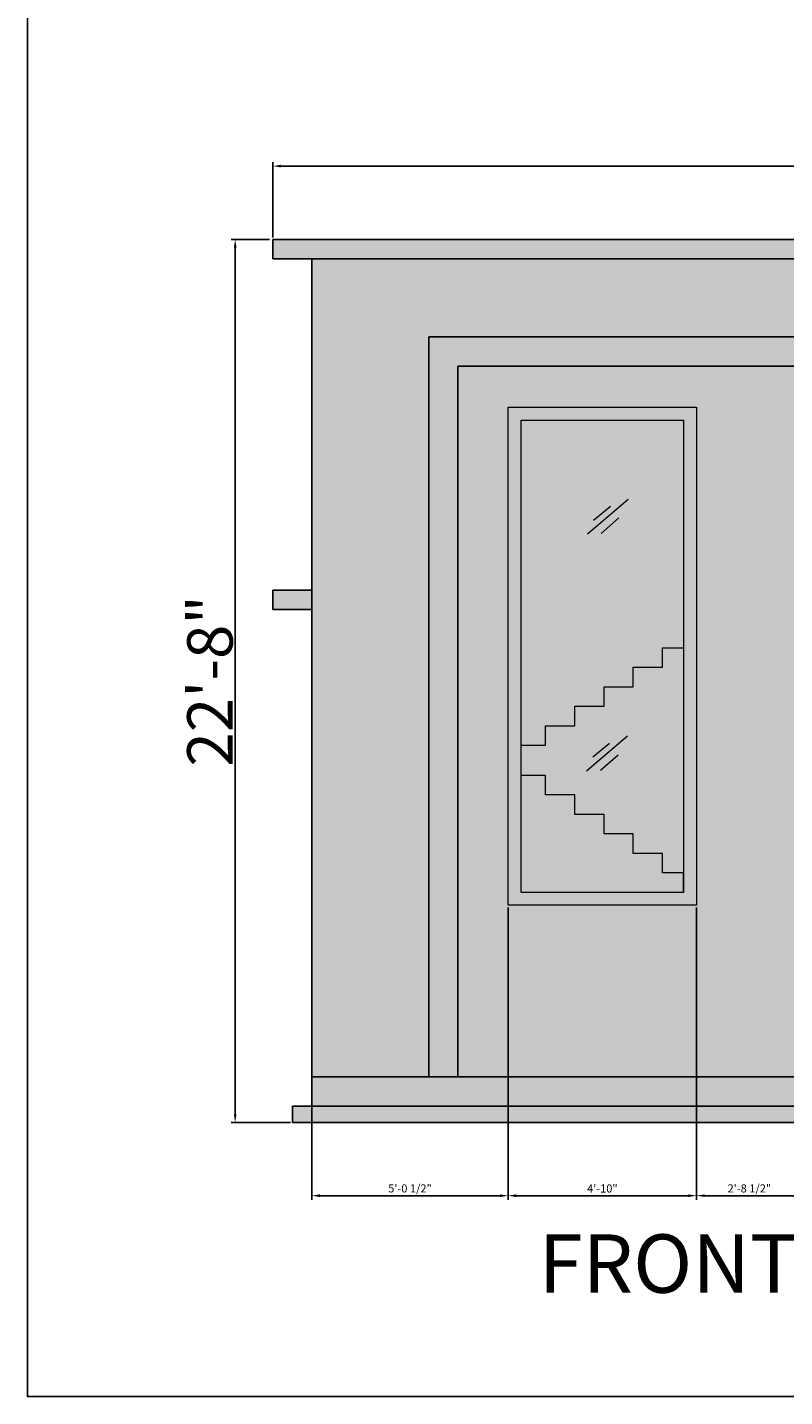
# Model space of a CAD drawing. Units: inches. Extents: x 2169 to 10664, y 1669 to 6352.
# Tile 1 of 17: x 2169 to 2403, y 1669 to 2091. Entities that reach past the tile are written whole.
import ezdxf

# ---------------------------------------------------------------- set-up
doc = ezdxf.new("R2010")
doc.units = ezdxf.units.IN
for name, color, linetype, lineweight in [('A-ANNO-DIMS', 3, 'Continuous', 18), ('A-ANNO-TITL', 3, 'Continuous', 25), ('A-ANNO-TTLB', 7, 'Continuous', 25), ('A-ELEV', 7, 'Continuous', 25), ('A-ELEV-CONC-PATT', 85, 'Continuous', 13), ('A-ELEV-OPEN', 7, 'Continuous', 18), ('A-ELEV-OPEN-PATT', 9, 'Continuous', 13), ('A-ELEV-PATT', 253, 'Continuous', 13), ('A-ELEV-STRS', 8, 'Continuous', 18)]:
    doc.layers.add(name, color=color, linetype=linetype, lineweight=lineweight)
doc.styles.get("Standard").update_dxf_attribs({"font": 'arial.ttf'})
doc.dimstyles.new('ISO-25', dxfattribs={"dimtxt": 2.5, "dimasz": 2.5, "dimexe": 1.25, "dimexo": 0.625, "dimtad": 1, "dimdec": 0, "dimlunit": 3, "dimtxsty": 'Standard', "dimcen": 2.5, "dimadec": 0, "dimazin": 0, "dimtfac": 1, "dimtdec": 0, "dimtmove": 0, "dimatfit": 3, "dimfxl": 1, "dimarcsym": 0})

# ---------------------------------------------------------------- blocks, each defined once
blk = doc.blocks.new('*D21')
at = {"layer": 'A-ANNO-DIMS', "color": 0, "lineweight": -2, "transparency": 16777216}
for p, q in [((2243.98, 2025.84), (2232.19, 2025.84)), ((2233.44, 2023.34), (2233.44, 1756.34)), ((2250.43, 1753.84), (2232.19, 1753.84))]:
    blk.add_line(p, q, dxfattribs=at)
at = {"layer": 'A-ANNO-DIMS', "color": 0, "transparency": 16777216}
for points in [[(2233.03, 2023.34), (2233.86, 2023.34), (2233.44, 2025.84)], [(2233.03, 1756.34), (2233.86, 1756.34), (2233.44, 1753.84)]]:
    blk.add_solid(points, dxfattribs=at)
at = {"layer": 'Defpoints', "color": 0, "transparency": 16777216}
for p in [(2244.61, 2025.84), (2233.44, 1753.84), (2251.06, 1753.84)]:
    blk.add_point(p, dxfattribs=at)
at = {"layer": 'A-ANNO-DIMS', "color": 0, "transparency": 16777216, "insert": (2225.67, 1889.84), "char_height": 2.5, "attachment_point": 5, "rotation": 90}
blk.add_mtext('{\\H5.6x;22\'-8"}', dxfattribs=at)
blk = doc.blocks.new('GLASS-MARK-A')
for p, q in [((0, 0), (12.55, 10.69)), ((1.85, 4.25), (7.07, 8.47)), ((4.25, 0.12), (9.7, 4.88))]:
    blk.add_line(p, q)
blk = doc.blocks.new('*D93')
at = {"layer": 'A-ANNO-DIMS', "color": 0, "lineweight": -2, "transparency": 16777216}
for p, q in [((2245.06, 2026.47), (2245.06, 2049.69)), ((2247.56, 2048.44), (2626.56, 2048.44)), ((2629.06, 2026.47), (2629.06, 2049.69))]:
    blk.add_line(p, q, dxfattribs=at)
at = {"layer": 'A-ANNO-DIMS', "color": 0, "transparency": 16777216}
for points in [[(2247.56, 2048.86), (2247.56, 2048.03), (2245.06, 2048.44)], [(2626.56, 2048.86), (2626.56, 2048.03), (2629.06, 2048.44)]]:
    blk.add_solid(points, dxfattribs=at)
at = {"layer": 'Defpoints', "color": 0, "transparency": 16777216}
for p in [(2629.06, 2048.44), (2245.06, 2025.84), (2629.06, 2025.84)]:
    blk.add_point(p, dxfattribs=at)
at = {"layer": 'A-ANNO-DIMS', "color": 0, "transparency": 16777216, "insert": (2437.06, 2050.35), "char_height": 2.5, "attachment_point": 5}
blk.add_mtext('32\'-0"', dxfattribs=at)
blk = doc.blocks.new('*D95')
at = {"layer": 'A-ANNO-DIMS', "color": 0, "lineweight": -2, "transparency": 16777216}
for p, q in [((2317.5, 1820.07), (2317.5, 1729.99)), ((2257.06, 1767.22), (2257.06, 1729.99)), ((2259.56, 1731.24), (2315, 1731.24))]:
    blk.add_line(p, q, dxfattribs=at)
at = {"layer": 'A-ANNO-DIMS', "color": 0, "transparency": 16777216}
for points in [[(2259.56, 1731.66), (2259.56, 1730.83), (2257.06, 1731.24)], [(2315, 1731.66), (2315, 1730.83), (2317.5, 1731.24)]]:
    blk.add_solid(points, dxfattribs=at)
at = {"layer": 'Defpoints', "color": 0, "transparency": 16777216}
for p in [(2317.5, 1820.7), (2257.06, 1767.84), (2317.5, 1731.24)]:
    blk.add_point(p, dxfattribs=at)
at = {"layer": 'A-ANNO-DIMS', "color": 0, "transparency": 16777216, "insert": (2287.28, 1733.16), "char_height": 2.5, "attachment_point": 5}
blk.add_mtext('5\'-0 1/2"', dxfattribs=at)
blk = doc.blocks.new('*D96')
at = {"layer": 'A-ANNO-DIMS', "color": 0, "lineweight": -2, "transparency": 16777216}
for p, q in [((2317.5, 1820.07), (2317.5, 1729.99)), ((2375.55, 1820.07), (2375.55, 1729.99)), ((2320, 1731.24), (2373.05, 1731.24))]:
    blk.add_line(p, q, dxfattribs=at)
at = {"layer": 'A-ANNO-DIMS', "color": 0, "transparency": 16777216}
for points in [[(2320, 1731.66), (2320, 1730.83), (2317.5, 1731.24)], [(2373.05, 1731.66), (2373.05, 1730.83), (2375.55, 1731.24)]]:
    blk.add_solid(points, dxfattribs=at)
at = {"layer": 'Defpoints', "color": 0, "transparency": 16777216}
for p in [(2317.5, 1820.7), (2375.55, 1820.7), (2375.55, 1731.24)]:
    blk.add_point(p, dxfattribs=at)
at = {"layer": 'A-ANNO-DIMS', "color": 0, "transparency": 16777216, "insert": (2346.52, 1733.14), "char_height": 2.5, "attachment_point": 5}
blk.add_mtext('4\'-10"', dxfattribs=at)
blk = doc.blocks.new('*D97')
at = {"layer": 'A-ANNO-DIMS', "color": 0, "lineweight": -2, "transparency": 16777216}
for p, q in [((2375.55, 1820.07), (2375.55, 1729.99)), ((2408.06, 1767.22), (2408.06, 1729.99)), ((2378.05, 1731.24), (2405.56, 1731.24))]:
    blk.add_line(p, q, dxfattribs=at)
at = {"layer": 'A-ANNO-DIMS', "color": 0, "transparency": 16777216}
for points in [[(2378.05, 1731.66), (2378.05, 1730.83), (2375.55, 1731.24)], [(2405.56, 1731.66), (2405.56, 1730.83), (2408.06, 1731.24)]]:
    blk.add_solid(points, dxfattribs=at)
at = {"layer": 'Defpoints', "color": 0, "transparency": 16777216}
for p in [(2375.55, 1820.7), (2408.06, 1767.84), (2408.06, 1731.24)]:
    blk.add_point(p, dxfattribs=at)
at = {"layer": 'A-ANNO-DIMS', "color": 0, "transparency": 16777216, "insert": (2391.8, 1733.16), "char_height": 2.5, "attachment_point": 5}
blk.add_mtext('2\'-8 1/2"', dxfattribs=at)

msp = doc.modelspace()

# ---------------------------------------------------------------- hatches: boundary and pattern name
at = {"layer": 'A-ELEV-CONC-PATT'}
h = msp.add_hatch(dxfattribs=at)
h.set_pattern_fill('AR-CONC', color=256, scale=0.02)
h.paths.add_polyline_path([(2629.06, 2025.84), (2245.06, 2025.84), (2245.06, 2019.84), (2629.06, 2019.84)])
h.paths.add_polyline_path([(2257.06, 1917.84), (2245.06, 1917.84), (2245.06, 1911.84), (2257.06, 1911.84)])
h.paths.add_polyline_path([(2629.06, 1917.84), (2408.06, 1917.84), (2408.06, 1911.84), (2629.06, 1911.84)])
h = msp.add_hatch(dxfattribs=at)
h.set_pattern_fill('AR-CONC', color=256, scale=0.02)
h.paths.add_polyline_path([(2408.06, 1995.84), (2293.06, 1995.84), (2293.06, 1767.84), (2302.06, 1767.84), (2302.06, 1986.84), (2408.06, 1986.84)])
at = {"layer": 'A-ELEV-OPEN-PATT'}
h = msp.add_hatch(color=256, dxfattribs=at)
h.dxf.hatch_style = 1
h.paths.add_polyline_path([(2375.55, 1974.13), (2317.5, 1974.13), (2317.5, 1820.7), (2375.55, 1820.7)])
h.paths.add_polyline_path([(2371.55, 1970.13), (2371.55, 1824.7), (2321.5, 1824.7), (2321.5, 1970.13)], flags=16)
h = msp.add_hatch(color=256, dxfattribs=at)
h.dxf.hatch_style = 1
h.paths.add_polyline_path([(2608.06, 1955.84), (2408.06, 1955.84), (2408.06, 1923.84), (2608.06, 1923.84)])
h.paths.add_polyline_path([(2371.55, 1970.13), (2321.5, 1970.13), (2321.5, 1870.03), (2329.06, 1870.03), (2329.06, 1876.03), (2338.06, 1876.03), (2338.06, 1882.03), (2347.06, 1882.03), (2347.06, 1888.03), (2356.06, 1888.03), (2356.06, 1894.03), (2365.06, 1894.03), (2365.06, 1900.03), (2371.55, 1900.03)])
h.paths.add_polyline_path([(2371.55, 1900.03), (2365.06, 1900.03), (2365.06, 1894.03), (2356.06, 1894.03), (2356.06, 1888.03), (2347.06, 1888.03), (2347.06, 1882.03), (2338.06, 1882.03), (2338.06, 1876.03), (2329.06, 1876.03), (2329.06, 1870.03), (2321.5, 1870.03), (2321.5, 1860.7), (2329.06, 1860.7), (2329.06, 1854.7), (2338.06, 1854.7), (2338.06, 1848.7), (2347.06, 1848.7), (2347.06, 1842.7), (2356.06, 1842.7), (2356.06, 1836.7), (2365.06, 1836.7), (2365.06, 1830.7), (2371.55, 1830.7)])
h.paths.add_polyline_path([(2365.06, 1836.7), (2356.06, 1836.7), (2356.06, 1842.7), (2347.06, 1842.7), (2347.06, 1848.7), (2338.06, 1848.7), (2338.06, 1854.7), (2329.06, 1854.7), (2329.06, 1860.7), (2321.5, 1860.7), (2321.5, 1824.7), (2371.55, 1824.7), (2371.55, 1830.7), (2365.06, 1830.7)])
at = {"layer": 'A-ELEV-PATT'}
h = msp.add_hatch(color=256, dxfattribs=at)
h.dxf.hatch_style = 1
h.paths.add_polyline_path([(2408.06, 1986.84), (2302.06, 1986.84), (2302.06, 1767.84), (2408.06, 1767.84)], flags=17)
h.paths.add_polyline_path([(2375.55, 1820.7), (2317.5, 1820.7), (2317.5, 1974.13), (2375.55, 1974.13)], flags=16)
h.paths.add_polyline_path([(2371.55, 1824.7), (2321.5, 1824.7), (2321.5, 1970.13), (2371.55, 1970.13)], flags=0)
h.paths.add_polyline_path([(2293.06, 1995.84), (2408.06, 1995.84), (2408.06, 2019.84), (2257.06, 2019.84), (2257.06, 1767.84), (2293.06, 1767.84)])
h = msp.add_hatch(color=256, dxfattribs=at)
h.dxf.hatch_style = 1
h.paths.add_polyline_path([(2617.06, 1767.84), (2257.06, 1767.84), (2257.06, 1758.84), (2617.06, 1758.84)])
h = msp.add_hatch(color=256, dxfattribs=at)
h.dxf.hatch_style = 1
h.paths.add_polyline_path([(2623.06, 1758.84), (2251.06, 1758.84), (2251.06, 1753.84), (2623.06, 1753.84)])

# ---------------------------------------------------------------- linework, layer by layer
at = {"layer": 'A-ANNO-TTLB'}
msp.add_lwpolyline([(2169.45, 2838.28), (3251.13, 2838.28), (3251.13, 1669.34), (2169.45, 1669.34)], close=True, dxfattribs=at)
at = {"layer": 'A-ELEV'}
for p, q in [((2245.06, 2025.84), (2629.06, 2025.84)), ((2245.06, 2019.84), (2245.06, 2025.84)), ((2245.06, 2019.84), (2629.06, 2019.84)), ((2257.06, 1758.84), (2257.06, 2019.84)), ((2293.06, 1767.84), (2293.06, 1995.84)), ((2293.06, 1995.84), (2408.06, 1995.84)), ((2302.06, 1767.84), (2302.06, 1986.84)), ((2302.06, 1986.84), (2408.06, 1986.84)), ((2257.06, 1917.84), (2245.06, 1917.84)), ((2245.06, 1911.84), (2245.06, 1917.84)), ((2245.06, 1911.84), (2245.06, 1917.84)), ((2257.06, 1911.84), (2245.06, 1911.84)), ((2257.06, 1767.84), (2617.06, 1767.84)), ((2251.06, 1758.84), (2623.06, 1758.84)), ((2251.06, 1753.84), (2251.06, 1758.84)), ((2251.06, 1753.84), (2623.06, 1753.84))]:
    msp.add_line(p, q, dxfattribs=at)
at = {"layer": 'A-ELEV-OPEN'}
for points in [[(2317.5, 1974.13), (2375.55, 1974.13), (2375.55, 1820.7), (2317.5, 1820.7)], [(2321.5, 1970.13), (2371.55, 1970.13), (2371.55, 1824.7), (2321.5, 1824.7)]]:
    msp.add_lwpolyline(points, close=True, dxfattribs=at)
at = {"layer": 'A-ELEV-STRS'}
for p, q in [((2321.5, 1897.42), (2321.5, 1903.42)), ((2365.06, 1894.03), (2365.06, 1900.03)), ((2365.06, 1900.03), (2371.55, 1900.03)), ((2356.06, 1888.03), (2356.06, 1894.03)), ((2356.06, 1894.03), (2365.06, 1894.03)), ((2347.06, 1882.03), (2347.06, 1888.03)), ((2347.06, 1888.03), (2356.06, 1888.03)), ((2338.06, 1876.03), (2338.06, 1882.03)), ((2338.06, 1882.03), (2347.06, 1882.03)), ((2329.06, 1870.03), (2329.06, 1876.03)), ((2329.06, 1876.03), (2338.06, 1876.03)), ((2321.5, 1870.03), (2329.06, 1870.03)), ((2329.06, 1860.7), (2321.5, 1860.7)), ((2329.06, 1854.7), (2329.06, 1860.7)), ((2338.06, 1854.7), (2329.06, 1854.7)), ((2338.06, 1848.7), (2338.06, 1854.7)), ((2347.06, 1848.7), (2338.06, 1848.7)), ((2347.06, 1842.7), (2347.06, 1848.7)), ((2356.06, 1842.7), (2347.06, 1842.7)), ((2356.06, 1836.7), (2356.06, 1842.7)), ((2365.06, 1836.7), (2356.06, 1836.7)), ((2365.06, 1830.7), (2365.06, 1836.7)), ((2371.55, 1830.7), (2365.06, 1830.7)), ((2371.55, 1824.7), (2371.55, 1830.7))]:
    msp.add_line(p, q, dxfattribs=at)

# ---------------------------------------------------------------- block references
at = {"layer": 'A-ELEV-OPEN'}
for p in [(2341.92, 1935.16), (2341.69, 1862.18)]:
    msp.add_blockref('GLASS-MARK-A', p, dxfattribs=at)

# ---------------------------------------------------------------- texts
at = {"layer": 'A-ANNO-TITL', "insert": (2326.86, 1719.32), "char_height": 18, "attachment_point": 1}
msp.add_mtext_dynamic_manual_height_columns('FRONT ELEVATION', width=700.4367, gutter_width=12.5, heights=[0], dxfattribs=at)

# ---------------------------------------------------------------- dimensions: what is measured, and where the dimension line sits
at = {"layer": 'A-ANNO-DIMS'}
for base, p1, p2, picture, middle in [((2629.06, 2048.44), (2245.06, 2025.84), (2629.06, 2025.84), '*D93', (2437.06, 2050.35)), ((2317.5, 1731.24), (2257.06, 1767.84), (2317.5, 1820.7), '*D95', (2287.28, 1733.16)), ((2375.5503, 1731.2434), (2317.4982, 1820.6968), (2375.5503, 1820.6968), '*D96', (2346.5242, 1733.1448)), ((2408.06, 1731.24), (2375.55, 1820.7), (2408.06, 1767.84), '*D97', (2391.8, 1733.16))]:
    dim = msp.add_linear_dim(base=base, p1=p1, p2=p2, dimstyle='ISO-25', override={"dimdec": 1, "dimlfac": 1, "dimrnd": 0, "dimzin": 1, "dimdsep": 46, "dimlunit": 4, "dimfrac": 2}, dxfattribs=at)
    dim.commit()
    dim.dimension.update_dxf_attribs({"geometry": picture, "text_midpoint": middle})
dim = msp.add_linear_dim(base=(2233.44, 1753.84), p1=(2244.61, 2025.84), p2=(2251.06, 1753.84), angle=90, text='{\\H5.6x;<>}', dimstyle='ISO-25', override={"dimclrd": 0, "dimclre": 0, "dimclrt": 0}, dxfattribs=at)
dim.commit()
dim.dimension.update_dxf_attribs({"geometry": '*D21', "text_midpoint": (2225.67, 1889.84)})

doc.saveas('drawing.dxf')
